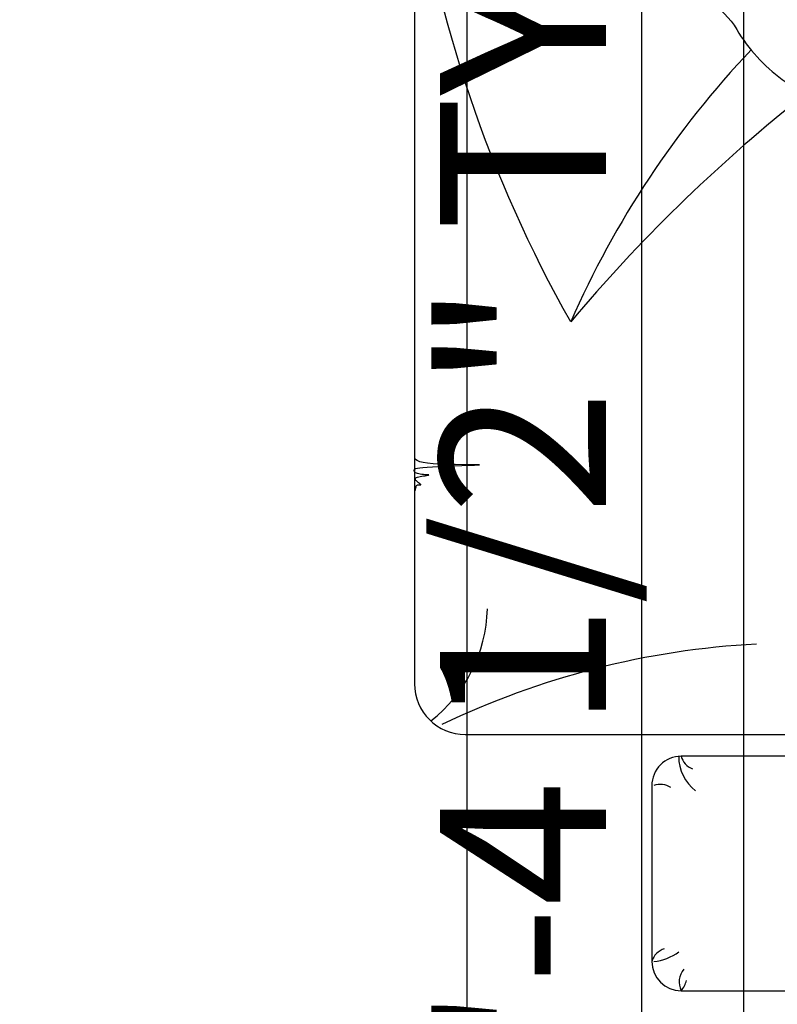
# Model space of a CAD drawing. Units: inches. Extents: x 3592 to 4861, y 1650 to 2243.
# Tile 21 of 30: x 4068 to 4109, y 2072 to 2125. Entities that reach past the tile are written whole.
import ezdxf

# ---------------------------------------------------------------- set-up
doc = ezdxf.new("R2010")
doc.units = ezdxf.units.IN
doc.layers.add('A-ANNO-DIMS', color=2, linetype='Continuous', lineweight=13)
doc.layers.add('A-FURN', color=9, linetype='Continuous', lineweight=13)
doc.layers.add('FUR', color=42, linetype='Continuous')
doc.styles.get("Standard").update_dxf_attribs({"font": 'arial.ttf'})
doc.dimstyles.new('ISO-25', dxfattribs={"dimtxt": 9, "dimasz": 2.5, "dimexe": 1.25, "dimexo": 0.625, "dimtad": 1, "dimlunit": 3, "dimtxsty": 'Standard', "dimcen": 2.5, "dimadec": 0, "dimazin": 0, "dimtfac": 1, "dimtmove": 0, "dimatfit": 3, "dimfxl": 1, "dimarcsym": 0})

# ---------------------------------------------------------------- blocks, each defined once
blk = doc.blocks.new('*X17')
at = {"color": 0}
for p, q in [((3163, 7776.2), (3163, 7776.2)), ((3422.2, 7761.3), (3422.2, 7761.3)), ((3244.3, 7698.6), (3244.3, 7698.6)), ((3340.3, 7689.4), (3340.3, 7689.4)), ((3236.2, 7675.7), (3236.2, 7675.7))]:
    blk.add_line(p, q, dxfattribs=at)
blk = doc.blocks.new('BED1')
for p, q in [((2187.2, 354.9), (2187.2, -545.1)), ((2587.2, -545.1), (2587.2, 354.9)), ((2237.2, -595.1), (2537.2, -595.1)), ((150, -1000), (2063.5, -1000))]:
    blk.add_line(p, q)
for points in [[(2150, -913.5), (2150, 723.2)], [(1733.7, -998.3), (1731.1, -998.1), (1729, -997.8), (1727.4, -997.4), (1726.1, -997), (1725.2, -996.4), (1724.7, -995.7), (1724.3, -994.8), (1724.1, -993.9), (1724.1, -992.9), (1724.1, -991.9), (1724.2, -991), (1724.2, -990.2), (1724.2, -989.7), (1724.1, -989.4), (1723.8, -989.5), (1723.2, -990), (1722.5, -990.8), (1721.7, -991.8), (1720.7, -993), (1719.7, -994.3), (1718.6, -995.5), (1717.5, -996.6), (1716.5, -997.6), (1715.5, -998.3), (1714.6, -998.6), (1713.8, -998.6), (1713, -998.3), (1712.3, -997.6), (1711.7, -996.5), (1711, -994.9), (1710.4, -992.9), (1709.9, -990.4), (1709.4, -987.6), (1708.9, -984.8), (1708.5, -982), (1708.1, -979.5), (1707.8, -977.4), (1707.5, -976.1), (1707.3, -975.5), (1707.1, -976), (1707, -977.3), (1706.9, -979.3), (1706.8, -981.8), (1706.7, -984.6), (1706.4, -987.5), (1706.1, -990.3), (1705.6, -992.9), (1705, -995.1), (1704.2, -996.9), (1703.4, -998.3), (1702.4, -999.3), (1701.5, -1000), (1700.5, -1000.4), (1699.6, -1000.6), (1698.7, -1000.4), (1697.8, -1000.1), (1697, -999.2), (1696.3, -997.6), (1695.7, -995), (1695.1, -991.1), (1694.5, -985.7), (1693.9, -978.5), (1693.3, -969.3), (1692.8, -957.9), (1692.2, -945.2), (1691.7, -931.9), (1691.2, -919), (1690.8, -907.4), (1690.4, -897.9), (1690.1, -891.5), (1689.9, -889.1), (1689.8, -891.2), (1689.8, -897.3), (1689.8, -906.5), (1689.7, -917.9), (1689.6, -930.6), (1689.4, -943.8), (1688.9, -956.6), (1688.3, -968.1), (1687.3, -977.6), (1686.1, -985.2), (1684.6, -991), (1682.8, -995.3), (1680.7, -998.3), (1679.6, -999.2)]]:
    blk.add_lwpolyline(points)
for points in [[(969.1, -259.1, 0.263265), (936.3, -236.9, -0.026108), (909.2, -233.2, 0.027613), (945.1, -234.2, -0.089259), (872.7, -120, 0.662242), (857.6, -119.3, -0.162037), (651.8, -332.7, 0.676499), (654, -354.5, -0.160513), (722.9, -401.5, 0.07473), (773.5, -450.3, -0.187721), (845.5, -559.9, 0.70791), (858.8, -561.4, -0.010003), (898.6, -497.3, -0.113819), (947.3, -450.2, 0.099539), (1032.5, -372.4, -0.173425), (1070.9, -346.4, 0.589988), (1076.2, -326.1, 0.137312), (923.9, -245.9, 0.137312)], [(1446, -733.4, -0.095039), (652.8, -1001.7)]]:
    blk.add_lwpolyline(points, format="xyb")
for centre, radius, start, end in [((3208.8, 1363.3), 2739.4, 218.6329, 229.9449), ((3402.5, -342.9), 1408.5, 182.9917, 205.6819), ((2098.7, 754.7), 1625, 226.5887, 246.3156), ((2188.1, -476.2), 73, 269.4513, 322.8027), ((2178, -513.5), 33, 286.1827, 338.1386), ((2562.2, -571.8), 36.5, 46.8095, 78.3841), ((2237.2, -545.1), 50, 180, 270), ((2453.3, -600), 84.5, 5.6196, 37.1396), ((2537.2, -545.1), 50, 270, 0), ((2572.5, -513.6), 34.8, 230.8413, 294.9586), ((2271.1, -580.9), 35.8, 148.9055, 197.5541), ((2546.9, -563.8), 32.8, 197.833, 252.8005), ((1929.1, -1126), 250.5, 37.8553, 88.4405), ((2063.5, -913.5), 86.5, 270, 0)]:
    blk.add_arc(centre, radius, start, end)
blk.add_blockref('*X17', (-2425.3, -8101.4))
blk = doc.blocks.new('A$C68AE1801')
at = {"layer": 'FUR', "xscale": 0.001, "yscale": 0.001, "zscale": 0.001, "rotation": 180}
blk.add_blockref('BED1', (2.5872, 1.49), dxfattribs=at)
blk = doc.blocks.new('*D150')
at = {"layer": 'A-ANNO-DIMS', "color": 0, "lineweight": -2, "transparency": 16777216}
for p, q in [((4101.85, 2020.278), (4101.85, 2140.684)), ((4100.037, 2020.278), (4103.1, 2020.278)), ((4101.85, 2006.522), (4101.85, 2017.778)), ((4100.037, 2004.022), (4103.1, 2004.022))]:
    blk.add_line(p, q, dxfattribs=at)
at = {"layer": 'A-ANNO-DIMS', "color": 0, "transparency": 16777216}
for points in [[(4101.433, 2017.778), (4102.267, 2017.778), (4101.85, 2020.278)], [(4101.433, 2006.522), (4102.267, 2006.522), (4101.85, 2004.022)]]:
    blk.add_solid(points, dxfattribs=at)
at = {"layer": 'Defpoints', "color": 0, "transparency": 16777216}
for p in [(4099.412, 2020.278), (4101.85, 2020.278), (4099.412, 2004.022)]:
    blk.add_point(p, dxfattribs=at)
at = {"layer": 'A-ANNO-DIMS', "color": 0, "transparency": 16777216, "insert": (4096.571, 2081.731), "char_height": 9, "attachment_point": 5, "rotation": 90}
blk.add_mtext('BASIN 1\'-4 1/2" TYP.', dxfattribs=at)
blk = doc.blocks.new('*D179')
at = {"layer": 'A-ANNO-DIMS', "color": 0, "lineweight": -2, "transparency": 16777216}
for p, q in [((4092.37, 2010.809), (4092.37, 2193.519)), ((4107.37, 2020.844), (4107.37, 2193.519)), ((4094.87, 2192.269), (4104.87, 2192.269)), ((4107.37, 2192.269), (4134.197, 2192.269))]:
    blk.add_line(p, q, dxfattribs=at)
at = {"layer": 'A-ANNO-DIMS', "color": 0, "transparency": 16777216}
for points in [[(4094.87, 2192.686), (4094.87, 2191.852), (4092.37, 2192.269)], [(4104.87, 2192.686), (4104.87, 2191.852), (4107.37, 2192.269)]]:
    blk.add_solid(points, dxfattribs=at)
at = {"layer": 'Defpoints', "color": 0, "transparency": 16777216}
for p in [(4107.37, 2192.269), (4107.37, 2020.219), (4092.37, 2010.184)]:
    blk.add_point(p, dxfattribs=at)
at = {"layer": 'A-ANNO-DIMS', "color": 0, "transparency": 16777216, "insert": (4122.033, 2197.492), "char_height": 9, "attachment_point": 5}
blk.add_mtext('1\'-3"', dxfattribs=at)

msp = doc.modelspace()

# ---------------------------------------------------------------- block references
at = {"layer": 'A-FURN', "xscale": 31.7658940618111, "yscale": 31.7658940618111, "zscale": 31.7658940618111, "rotation": 90}
msp.add_blockref('A$C68AE1801', (4168.621, 2072.607), dxfattribs=at)

# ---------------------------------------------------------------- dimensions: what is measured, and where the dimension line sits
at = {"layer": 'A-ANNO-DIMS'}
dim = msp.add_linear_dim(base=(4107.37, 2192.269), p1=(4092.37, 2010.184), p2=(4107.37, 2020.219), dimstyle='ISO-25', override={"dimdec": 1, "dimlfac": 1, "dimrnd": 0, "dimzin": 1, "dimdsep": 46, "dimlunit": 4, "dimfrac": 2}, dxfattribs=at)
dim.commit()
dim.dimension.update_dxf_attribs({"geometry": '*D179', "text_midpoint": (4122.033, 2197.492)})
dim = msp.add_linear_dim(base=(4101.85, 2020.278), p1=(4099.412, 2004.022), p2=(4099.412, 2020.278), angle=90, text='BASIN <> TYP.', dimstyle='ISO-25', override={"dimdec": 1, "dimlfac": 1, "dimrnd": 0, "dimzin": 1, "dimdsep": 46, "dimlunit": 4, "dimfrac": 2}, dxfattribs=at)
dim.commit()
dim.dimension.update_dxf_attribs({"geometry": '*D150', "text_midpoint": (4096.571, 2081.731)})

doc.saveas('drawing.dxf')
